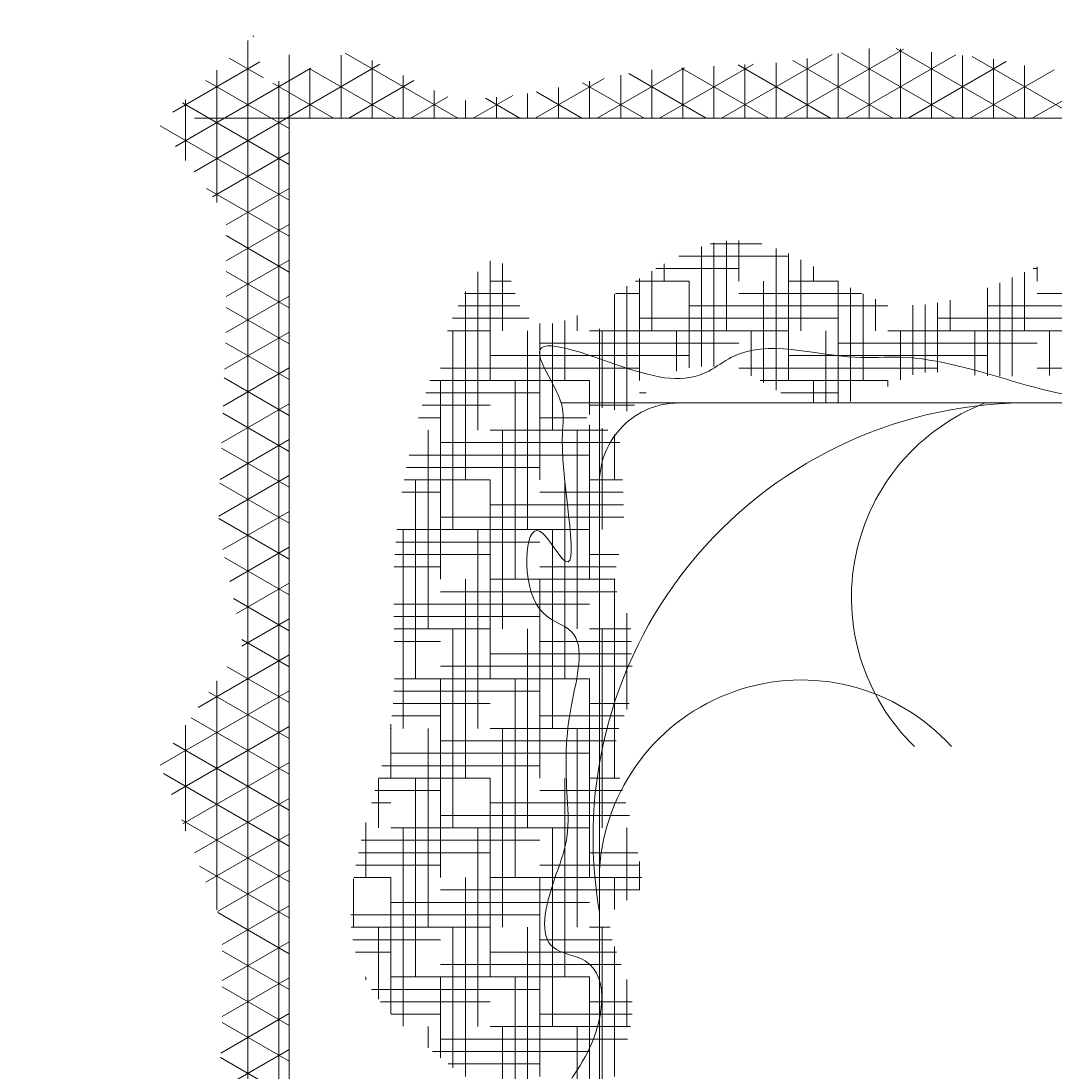
# Model space of a CAD drawing. Units: inches. Extents: x 3731 to 4318, y 1310 to 2388.
# Tile 44 of 57: x 4124 to 4167, y 1999 to 2043. Entities that reach past the tile are written whole.
import ezdxf

# ---------------------------------------------------------------- set-up
doc = ezdxf.new("R2010")
doc.units = ezdxf.units.IN
doc.layers.add('A-ANNO-DIMS', color=2, linetype='Continuous', lineweight=18)
doc.layers.add('A-FURN', color=8, linetype='Continuous', lineweight=13)
doc.styles.get("Standard").update_dxf_attribs({"font": 'arial.ttf'})
doc.dimstyles.get("Standard").update_dxf_attribs({"dimtxt": 0.18, "dimasz": 0.18, "dimexe": 0.18, "dimexo": 0.0625, "dimgap": 0.09, "dimtad": 0, "dimtih": 1, "dimtoh": 1, "dimdec": 4, "dimzin": 0, "dimdsep": 46, "dimtxsty": 'Standard', "dimcen": 0.09, "dimadec": 0, "dimazin": 0, "dimtfac": 1, "dimtdec": 4, "dimtofl": 0, "dimtmove": 0, "dimatfit": 3, "dimfxl": 1, "dimtolj": 1, "dimtzin": 0, "dimarcsym": 0})

# ---------------------------------------------------------------- blocks, each defined once
blk = doc.blocks.new('A$C200C7901')
for p, q in [((2.3121, 1.6596), (2.3121, 0.0201)), ((2, 0.2957), (2, 1.2957)), ((2.0224, 0.9977), (2.0224, 1.1977)), ((2.0224, 0.9977), (2.0224, 1.1977)), ((1.9974, 0.5977), (1.9974, 0.7977)), ((1.9974, 0.5977), (1.9974, 0.7977)), ((2.0724, 0.5977), (2.0724, 0.7977)), ((2.0724, 0.5977), (2.0724, 0.7977)), ((2.1474, 0.5977), (2.1474, 0.7977)), ((2.1474, 0.5977), (2.1474, 0.7977)), ((1.9849, 0.5477), (1.9849, 0.7477)), ((1.9849, 0.5477), (1.9849, 0.7477)), ((2.0599, 0.5477), (2.0599, 0.7477)), ((2.0599, 0.5477), (2.0599, 0.7477)), ((2.1349, 0.5477), (2.1349, 0.7477)), ((2.1349, 0.5477), (2.1349, 0.7477)), ((0.4061, 0.3703), (2.0386, 0.3703)), ((2.4073, 0.0839), (0.9625, 0.0839))]:
    blk.add_line(p, q)
at = {"linetype": 'ByBlock'}
for p, q in [((2.3224, 0.0468), (2.3224, 1.6627)), ((2.3224, 0.0468), (2.3224, 1.6627)), ((2.3537, 0.0056), (2.3537, 1.634)), ((2.3537, 0.0056), (2.3537, 1.634)), ((2.0099, 0.9477), (2.0099, 1.1477)), ((2.0099, 0.9477), (2.0099, 1.1477)), ((2.0849, 0.9477), (2.0849, 1.1477)), ((2.0849, 0.9477), (2.0849, 1.1477)), ((1.9974, 0.8977), (1.9974, 1.0977)), ((1.9974, 0.8977), (1.9974, 1.0977)), ((2.0724, 0.8977), (2.0724, 1.0977)), ((2.0724, 0.8977), (2.0724, 1.0977)), ((2.0974, 0.9977), (2.0974, 1.0909)), ((2.0974, 0.9977), (2.0974, 1.0909)), ((2.3121, 1.0686), (2.3813, 1.0286)), ((2.3121, 1.0686), (2.3813, 1.0286)), ((2.3121, 1.0206), (2.3851, 1.0628)), ((2.3121, 1.0206), (2.3851, 1.0628)), ((1.9849, 0.9171), (1.9849, 1.0477)), ((1.9849, 0.9171), (1.9849, 1.0477)), ((2.0599, 0.8477), (2.0599, 1.0477)), ((2.0599, 0.8477), (2.0599, 1.0477)), ((2.1349, 0.8477), (2.1349, 1.0477)), ((2.1349, 0.8477), (2.1349, 1.0477)), ((2.0599, 1.0352), (2.1523, 1.0352)), ((2.0599, 1.0352), (2.1523, 1.0352)), ((2.1474, 0.8977), (2.1474, 1.0391)), ((2.1474, 0.8977), (2.1474, 1.0391)), ((2.1599, 0.9477), (2.1599, 1.029)), ((2.1599, 0.9477), (2.1599, 1.029)), ((2.3121, 1.0325), (2.3795, 0.9936)), ((2.3121, 1.0325), (2.3795, 0.9936)), ((2.0099, 1.0227), (2.1678, 1.0227)), ((2.0099, 1.0227), (2.1678, 1.0227)), ((2.1724, 0.9977), (2.1724, 1.0189)), ((2.1724, 0.9977), (2.1724, 1.0189)), ((2.3121, 0.9846), (2.3809, 1.0242)), ((2.3121, 0.9846), (2.3809, 1.0242)), ((1.9718, 1.0102), (2.1599, 1.0102)), ((1.9718, 1.0102), (2.1599, 1.0102)), ((1.9688, 0.9977), (2.1099, 0.9977)), ((1.9688, 0.9977), (2.1099, 0.9977)), ((1.9724, 0.9504), (1.9724, 0.9977)), ((1.9724, 0.9504), (1.9724, 0.9977)), ((2.0474, 0.7977), (2.0474, 0.9977)), ((2.0474, 0.7977), (2.0474, 0.9977)), ((2.1224, 0.7977), (2.1224, 0.9977)), ((2.1224, 0.7977), (2.1224, 0.9977)), ((2.1974, 0.7977), (2.1974, 0.9972)), ((2.1974, 0.7977), (2.1974, 0.9972)), ((2.3121, 0.9964), (2.3795, 0.9575)), ((2.3121, 0.9964), (2.3795, 0.9575)), ((1.9671, 0.9852), (2.0599, 0.9852)), ((1.9671, 0.9852), (2.0599, 0.9852)), ((2.1599, 0.9852), (2.2095, 0.9852)), ((2.1599, 0.9852), (2.2095, 0.9852)), ((2.2099, 0.8477), (2.2099, 0.9848)), ((2.2099, 0.8477), (2.2099, 0.9848)), ((2.3121, 0.9485), (2.3795, 0.9874)), ((2.3121, 0.9485), (2.3795, 0.9874)), ((1.9672, 0.9727), (2.0099, 0.9727)), ((1.9672, 0.9727), (2.0099, 0.9727)), ((2.1099, 0.9727), (2.2204, 0.9727)), ((2.1099, 0.9727), (2.2204, 0.9727)), ((2.2224, 0.8977), (2.2224, 0.9702)), ((2.2224, 0.8977), (2.2224, 0.9702)), ((2.0599, 0.9602), (2.2294, 0.9602)), ((2.0599, 0.9602), (2.2294, 0.9602)), ((2.2349, 0.9477), (2.2349, 0.9506)), ((2.2349, 0.9477), (2.2349, 0.9506)), ((2.3121, 0.9603), (2.3795, 0.9215)), ((2.3121, 0.9603), (2.3795, 0.9215)), ((2.3121, 0.9124), (2.3795, 0.9513)), ((2.3121, 0.9124), (2.3795, 0.9513)), ((2.0099, 0.9477), (2.2099, 0.9477)), ((2.0099, 0.9477), (2.2099, 0.9477)), ((2.0349, 0.7477), (2.0349, 0.9477)), ((2.0349, 0.7477), (2.0349, 0.9477)), ((2.1099, 0.7477), (2.1099, 0.9477)), ((2.1099, 0.7477), (2.1099, 0.9477)), ((2.1849, 0.7477), (2.1849, 0.9477)), ((2.1849, 0.7477), (2.1849, 0.9477)), ((1.9781, 0.9352), (2.1599, 0.9352)), ((1.9781, 0.9352), (2.1599, 0.9352)), ((1.9829, 0.9227), (2.1099, 0.9227)), ((1.9829, 0.9227), (2.1099, 0.9227)), ((2.2099, 0.9227), (2.2455, 0.9227)), ((2.2099, 0.9227), (2.2455, 0.9227)), ((2.3121, 0.9243), (2.3838, 0.8829)), ((2.3121, 0.9243), (2.3838, 0.8829)), ((1.9871, 0.9102), (2.0599, 0.9102)), ((1.9871, 0.9102), (2.0599, 0.9102)), ((2.1599, 0.9102), (2.2481, 0.9102)), ((2.1599, 0.9102), (2.2481, 0.9102)), ((2.3121, 0.8763), (2.3795, 0.9152)), ((2.3121, 0.8763), (2.3795, 0.9152)), ((1.9894, 0.8977), (2.0099, 0.8977)), ((1.9894, 0.8977), (2.0099, 0.8977)), ((2.0224, 0.6977), (2.0224, 0.8977)), ((2.0224, 0.6977), (2.0224, 0.8977)), ((2.0974, 0.6977), (2.0974, 0.8977)), ((2.0974, 0.6977), (2.0974, 0.8977)), ((2.1099, 0.8977), (2.2496, 0.8977)), ((2.1099, 0.8977), (2.2496, 0.8977)), ((2.1724, 0.6977), (2.1724, 0.8977)), ((2.1724, 0.6977), (2.1724, 0.8977)), ((2.2474, 0.8489), (2.2474, 0.8977)), ((2.2474, 0.8489), (2.2474, 0.8977)), ((2.3121, 0.8882), (2.4022, 0.8362)), ((2.3121, 0.8882), (2.4022, 0.8362)), ((1.9849, 0.8477), (1.9849, 0.88)), ((1.9849, 0.8477), (1.9849, 0.88)), ((2.0599, 0.8852), (2.2501, 0.8852)), ((2.0599, 0.8852), (2.2501, 0.8852)), ((2.3121, 0.8402), (2.3842, 0.8818)), ((2.3121, 0.8402), (2.3842, 0.8818)), ((2.3849, 0.6497), (2.3849, 0.8801)), ((2.3849, 0.6497), (2.3849, 0.8801)), ((1.9724, 0.7977), (1.9724, 0.8703)), ((1.9724, 0.7977), (1.9724, 0.8703)), ((2.0099, 0.8727), (2.2099, 0.8727)), ((2.0099, 0.8727), (2.2099, 0.8727)), ((1.9599, 0.8317), (1.9599, 0.8604)), ((1.9599, 0.8317), (1.9599, 0.8604)), ((1.9599, 0.8602), (2.1599, 0.8602)), ((1.9599, 0.8602), (2.1599, 0.8602)), ((1.9574, 0.8477), (2.1099, 0.8477)), ((1.9574, 0.8477), (2.1099, 0.8477)), ((2.0099, 0.6477), (2.0099, 0.8477)), ((2.0099, 0.6477), (2.0099, 0.8477)), ((2.0849, 0.6477), (2.0849, 0.8477)), ((2.0849, 0.6477), (2.0849, 0.8477)), ((2.1599, 0.6477), (2.1599, 0.8477)), ((2.1599, 0.6477), (2.1599, 0.8477)), ((2.2099, 0.8477), (2.2472, 0.8477)), ((2.2099, 0.8477), (2.2472, 0.8477)), ((2.2349, 0.7923), (2.2349, 0.8477)), ((2.2349, 0.7923), (2.2349, 0.8477)), ((2.3121, 0.8041), (2.3958, 0.8524)), ((2.3121, 0.8041), (2.3958, 0.8524)), ((2.3121, 0.8521), (2.4205, 0.7895)), ((2.3121, 0.8521), (2.4205, 0.7895)), ((1.9593, 0.8352), (2.0599, 0.8352)), ((1.9593, 0.8352), (2.0599, 0.8352)), ((2.1599, 0.8352), (2.2451, 0.8352)), ((2.1599, 0.8352), (2.2451, 0.8352)), ((1.9615, 0.8227), (2.0099, 0.8227)), ((1.9615, 0.8227), (2.0099, 0.8227)), ((2.1099, 0.8227), (2.2425, 0.8227)), ((2.1099, 0.8227), (2.2425, 0.8227)), ((2.3121, 0.7681), (2.4073, 0.823)), ((2.3121, 0.7681), (2.4073, 0.823)), ((2.3121, 0.816), (2.4384, 0.7431)), ((2.3121, 0.816), (2.4384, 0.7431)), ((2.0599, 0.8102), (2.2396, 0.8102)), ((2.0599, 0.8102), (2.2396, 0.8102)), ((2.0099, 0.7977), (2.2099, 0.7977)), ((2.0099, 0.7977), (2.2099, 0.7977)), ((2.2224, 0.7483), (2.2224, 0.7977)), ((2.2224, 0.7483), (2.2224, 0.7977)), ((2.3121, 0.732), (2.4189, 0.7936)), ((2.3121, 0.732), (2.4189, 0.7936)), ((2.4162, 0.6946), (2.4162, 0.8006)), ((2.4162, 0.6946), (2.4162, 0.8006)), ((1.9699, 0.7852), (2.1599, 0.7852)), ((1.9699, 0.7852), (2.1599, 0.7852)), ((1.9734, 0.7727), (2.1099, 0.7727)), ((1.9734, 0.7727), (2.1099, 0.7727)), ((2.2099, 0.7727), (2.2294, 0.7727)), ((2.2099, 0.7727), (2.2294, 0.7727)), ((2.3121, 0.7799), (2.4287, 0.7126)), ((2.3121, 0.7799), (2.4287, 0.7126)), ((2.3121, 0.6959), (2.4303, 0.7641)), ((2.3121, 0.6959), (2.4303, 0.7641)), ((1.9767, 0.7602), (2.0599, 0.7602)), ((1.9767, 0.7602), (2.0599, 0.7602)), ((2.1599, 0.7602), (2.2258, 0.7602)), ((2.1599, 0.7602), (2.2258, 0.7602)), ((1.9797, 0.7477), (2.0099, 0.7477)), ((1.9797, 0.7477), (2.0099, 0.7477)), ((2.1099, 0.7477), (2.2222, 0.7477)), ((2.1099, 0.7477), (2.2222, 0.7477)), ((2.2099, 0.6933), (2.2099, 0.7477)), ((2.2099, 0.6933), (2.2099, 0.7477)), ((2.3121, 0.7438), (2.4108, 0.6869)), ((2.3121, 0.7438), (2.4108, 0.6869)), ((2.0599, 0.7352), (2.2188, 0.7352)), ((2.0599, 0.7352), (2.2188, 0.7352)), ((2.3121, 0.6598), (2.4417, 0.7346)), ((2.3121, 0.6598), (2.4417, 0.7346)), ((2.0099, 0.7227), (2.2099, 0.7227)), ((2.0099, 0.7227), (2.2099, 0.7227)), ((1.9831, 0.7102), (2.1599, 0.7102)), ((1.9831, 0.7102), (2.1599, 0.7102)), ((2.3121, 0.7078), (2.3929, 0.6611)), ((2.3121, 0.7078), (2.3929, 0.6611)), ((1.9804, 0.6977), (2.1099, 0.6977)), ((1.9804, 0.6977), (2.1099, 0.6977)), ((2.0474, 0.4977), (2.0474, 0.6977)), ((2.0474, 0.4977), (2.0474, 0.6977)), ((2.1224, 0.4977), (2.1224, 0.6977)), ((2.1224, 0.4977), (2.1224, 0.6977)), ((2.1974, 0.4977), (2.1974, 0.6977)), ((2.1974, 0.4977), (2.1974, 0.6977)), ((2.2099, 0.6977), (2.2106, 0.6977)), ((2.2099, 0.6977), (2.2106, 0.6977)), ((1.9724, 0.5818), (1.9724, 0.6786)), ((1.9724, 0.5818), (1.9724, 0.6786)), ((1.9753, 0.6852), (2.0599, 0.6852)), ((1.9753, 0.6852), (2.0599, 0.6852)), ((2.1599, 0.6852), (2.2088, 0.6852)), ((2.1599, 0.6852), (2.2088, 0.6852)), ((2.3121, 0.6237), (2.4036, 0.6765)), ((2.3121, 0.6237), (2.4036, 0.6765)), ((1.97, 0.6727), (2.0099, 0.6727)), ((1.97, 0.6727), (2.0099, 0.6727)), ((2.1099, 0.6727), (2.2075, 0.6727)), ((2.1099, 0.6727), (2.2075, 0.6727)), ((2.3121, 0.6717), (2.3744, 0.6357)), ((2.3121, 0.6717), (2.3744, 0.6357)), ((2.0599, 0.6602), (2.2067, 0.6602)), ((2.0599, 0.6602), (2.2067, 0.6602)), ((2.0099, 0.6477), (2.2062, 0.6477)), ((2.0099, 0.6477), (2.2062, 0.6477)), ((2.0349, 0.4477), (2.0349, 0.6477)), ((2.0349, 0.4477), (2.0349, 0.6477)), ((2.1099, 0.4477), (2.1099, 0.6477)), ((2.1099, 0.4477), (2.1099, 0.6477)), ((2.1849, 0.4477), (2.1849, 0.6477)), ((2.1849, 0.4477), (2.1849, 0.6477)), ((1.9673, 0.6352), (2.1599, 0.6352)), ((1.9673, 0.6352), (2.1599, 0.6352)), ((2.3121, 0.6356), (2.3598, 0.6081)), ((2.3121, 0.6356), (2.3598, 0.6081)), ((1.9678, 0.6227), (2.1099, 0.6227)), ((1.9678, 0.6227), (2.1099, 0.6227)), ((2.3121, 0.5876), (2.3598, 0.6151)), ((2.3121, 0.5876), (2.3598, 0.6151)), ((1.9679, 0.6102), (2.0599, 0.6102)), ((1.9679, 0.6102), (2.0599, 0.6102)), ((2.1599, 0.6102), (2.2064, 0.6102)), ((2.1599, 0.6102), (2.2064, 0.6102)), ((1.9685, 0.5977), (2.0099, 0.5977)), ((1.9685, 0.5977), (2.0099, 0.5977)), ((2.0224, 0.3977), (2.0224, 0.5977)), ((2.0224, 0.3977), (2.0224, 0.5977)), ((2.0974, 0.3977), (2.0974, 0.5977)), ((2.0974, 0.3977), (2.0974, 0.5977)), ((2.1099, 0.5977), (2.2066, 0.5977)), ((2.1099, 0.5977), (2.2066, 0.5977)), ((2.1724, 0.3977), (2.1724, 0.5977)), ((2.1724, 0.3977), (2.1724, 0.5977)), ((2.3121, 0.5995), (2.3682, 0.5671)), ((2.3121, 0.5995), (2.3682, 0.5671)), ((2.0599, 0.5852), (2.2069, 0.5852)), ((2.0599, 0.5852), (2.2069, 0.5852)), ((2.3121, 0.5515), (2.365, 0.5821)), ((2.3121, 0.5515), (2.365, 0.5821)), ((2.0099, 0.5727), (2.207, 0.5727)), ((2.0099, 0.5727), (2.207, 0.5727)), ((1.9827, 0.5602), (2.1599, 0.5602)), ((1.9827, 0.5602), (2.1599, 0.5602)), ((2.3121, 0.5634), (2.3771, 0.5259)), ((2.3121, 0.5634), (2.3771, 0.5259)), ((2.3121, 0.5155), (2.3719, 0.55)), ((2.3121, 0.5155), (2.3719, 0.55)), ((1.9842, 0.5477), (2.1099, 0.5477)), ((1.9842, 0.5477), (2.1099, 0.5477)), ((2.0099, 0.3923), (2.0099, 0.5477)), ((2.0099, 0.3923), (2.0099, 0.5477)), ((2.0849, 0.3477), (2.0849, 0.5477)), ((2.0849, 0.3477), (2.0849, 0.5477)), ((2.1599, 0.3477), (2.1599, 0.5477)), ((2.1599, 0.3477), (2.1599, 0.5477)), ((1.9831, 0.5352), (2.0599, 0.5352)), ((1.9831, 0.5352), (2.0599, 0.5352)), ((2.1599, 0.5352), (2.2065, 0.5352)), ((2.1599, 0.5352), (2.2065, 0.5352)), ((1.9807, 0.5227), (2.0099, 0.5227)), ((1.9807, 0.5227), (2.0099, 0.5227)), ((2.1099, 0.5227), (2.2058, 0.5227)), ((2.1099, 0.5227), (2.2058, 0.5227)), ((2.3121, 0.5273), (2.383, 0.4864)), ((2.3121, 0.5273), (2.383, 0.4864)), ((2.3121, 0.4794), (2.3788, 0.5179)), ((2.3121, 0.4794), (2.3788, 0.5179)), ((2.0599, 0.5102), (2.2049, 0.5102)), ((2.0599, 0.5102), (2.2049, 0.5102)), ((1.9974, 0.3957), (1.9974, 0.4977)), ((1.9974, 0.3957), (1.9974, 0.4977)), ((2.0099, 0.4977), (2.2038, 0.4977)), ((2.0099, 0.4977), (2.2038, 0.4977)), ((2.0724, 0.2977), (2.0724, 0.4977)), ((2.0724, 0.2977), (2.0724, 0.4977)), ((2.1474, 0.2977), (2.1474, 0.4977)), ((2.1474, 0.2977), (2.1474, 0.4977)), ((2.3121, 0.4912), (2.3817, 0.4511)), ((2.3121, 0.4912), (2.3817, 0.4511)), ((1.9755, 0.4852), (2.1599, 0.4852)), ((1.9755, 0.4852), (2.1599, 0.4852)), ((2.3121, 0.4433), (2.383, 0.4842)), ((2.3121, 0.4433), (2.383, 0.4842)), ((1.9757, 0.4727), (2.1099, 0.4727)), ((1.9757, 0.4727), (2.1099, 0.4727)), ((1.9762, 0.4602), (2.0599, 0.4602)), ((1.9762, 0.4602), (2.0599, 0.4602)), ((2.1599, 0.4602), (2.1987, 0.4602)), ((2.1599, 0.4602), (2.1987, 0.4602)), ((2.3121, 0.4552), (2.3803, 0.4158)), ((2.3121, 0.4552), (2.3803, 0.4158)), ((1.9768, 0.4477), (2.0099, 0.4477)), ((1.9768, 0.4477), (2.0099, 0.4477)), ((1.9849, 0.402), (1.9849, 0.4477)), ((1.9849, 0.402), (1.9849, 0.4477)), ((2.0599, 0.2903), (2.0599, 0.4477)), ((2.0599, 0.2903), (2.0599, 0.4477)), ((2.1099, 0.4477), (2.1965, 0.4477)), ((2.1099, 0.4477), (2.1965, 0.4477)), ((2.1349, 0.2582), (2.1349, 0.4477)), ((2.1349, 0.2582), (2.1349, 0.4477)), ((2.3121, 0.4072), (2.3815, 0.4473)), ((2.3121, 0.4072), (2.3815, 0.4473)), ((2.0599, 0.4352), (2.194, 0.4352)), ((2.0599, 0.4352), (2.194, 0.4352)), ((2.0099, 0.4227), (2.1913, 0.4227)), ((2.0099, 0.4227), (2.1913, 0.4227)), ((2.3121, 0.4191), (2.3789, 0.3805)), ((2.3121, 0.4191), (2.3789, 0.3805)), ((1.9797, 0.4102), (2.1599, 0.4102)), ((1.9797, 0.4102), (2.1599, 0.4102)), ((2.3121, 0.3711), (2.3801, 0.4103)), ((2.3121, 0.3711), (2.3801, 0.4103)), ((1.9915, 0.3977), (2.1099, 0.3977)), ((1.9915, 0.3977), (2.1099, 0.3977)), ((2.0474, 0.2905), (2.0474, 0.3977)), ((2.0474, 0.2905), (2.0474, 0.3977)), ((2.1224, 0.2385), (2.1224, 0.3977)), ((2.1224, 0.2385), (2.1224, 0.3977)), ((2.0099, 0.3477), (2.0099, 0.382)), ((2.0099, 0.3477), (2.0099, 0.382)), ((2.0127, 0.3852), (2.0599, 0.3852)), ((2.0127, 0.3852), (2.0599, 0.3852)), ((2.1599, 0.3852), (2.1819, 0.3852)), ((2.1599, 0.3852), (2.1819, 0.3852)), ((2.3121, 0.383), (2.3775, 0.3452)), ((2.3121, 0.383), (2.3775, 0.3452)), ((1.7599, 0.2477), (1.7599, 0.3703)), ((1.7599, 0.2477), (1.7599, 0.3703)), ((1.7724, 0.2977), (1.7724, 0.3703)), ((1.7724, 0.2977), (1.7724, 0.3703)), ((1.7849, 0.3477), (1.7849, 0.3703)), ((1.7849, 0.3477), (1.7849, 0.3703)), ((1.9648, 0.3727), (2.0099, 0.3727)), ((1.9648, 0.3727), (2.0099, 0.3727)), ((1.9724, 0.253), (1.9724, 0.3785)), ((1.9724, 0.253), (1.9724, 0.3785)), ((1.9849, 0.2609), (1.9849, 0.3774)), ((1.9849, 0.2609), (1.9849, 0.3774)), ((1.9974, 0.2977), (1.9974, 0.3753)), ((1.9974, 0.2977), (1.9974, 0.3753)), ((2.1099, 0.3727), (2.1784, 0.3727)), ((2.1099, 0.3727), (2.1784, 0.3727)), ((2.3121, 0.335), (2.3786, 0.3734)), ((2.3121, 0.335), (2.3786, 0.3734)), ((1.7474, 0.2546), (1.7474, 0.3689)), ((1.7474, 0.2546), (1.7474, 0.3689)), ((1.7599, 0.3602), (1.8177, 0.3602)), ((1.7599, 0.3602), (1.8177, 0.3602)), ((1.9532, 0.3602), (1.9599, 0.3602)), ((1.9532, 0.3602), (1.9599, 0.3602)), ((2.0599, 0.3602), (2.1747, 0.3602)), ((2.0599, 0.3602), (2.1747, 0.3602)), ((1.7099, 0.3477), (1.7099, 0.3539)), ((1.7099, 0.3477), (1.7099, 0.3539)), ((1.8224, 0.2148), (1.8224, 0.3575)), ((1.8224, 0.2148), (1.8224, 0.3575)), ((1.8349, 0.2477), (1.8349, 0.3497)), ((1.8349, 0.2477), (1.8349, 0.3497)), ((1.5474, 0.2977), (1.5474, 0.3428)), ((1.5474, 0.2977), (1.5474, 0.3428)), ((1.5849, 0.2443), (1.5849, 0.3434)), ((1.5849, 0.2443), (1.5849, 0.3434)), ((1.5974, 0.2496), (1.5974, 0.3435)), ((1.5974, 0.2496), (1.5974, 0.3435)), ((1.6099, 0.2546), (1.6099, 0.3432)), ((1.6099, 0.2546), (1.6099, 0.3432)), ((1.6224, 0.2977), (1.6224, 0.3424)), ((1.6224, 0.2977), (1.6224, 0.3424)), ((1.6599, 0.2695), (1.6599, 0.3394)), ((1.6599, 0.2695), (1.6599, 0.3394)), ((1.6724, 0.2713), (1.6724, 0.3398)), ((1.6724, 0.2713), (1.6724, 0.3398)), ((1.6849, 0.272), (1.6849, 0.3422)), ((1.6849, 0.272), (1.6849, 0.3422)), ((1.6974, 0.2977), (1.6974, 0.3472)), ((1.6974, 0.2977), (1.6974, 0.3472)), ((1.7099, 0.3477), (1.8383, 0.3477)), ((1.7099, 0.3477), (1.8383, 0.3477)), ((1.7349, 0.2607), (1.7349, 0.3477)), ((1.7349, 0.2607), (1.7349, 0.3477)), ((1.8099, 0.2201), (1.8099, 0.3477)), ((1.8099, 0.2201), (1.8099, 0.3477)), ((1.8474, 0.2977), (1.8474, 0.3432)), ((1.8474, 0.2977), (1.8474, 0.3432)), ((1.9224, 0.2977), (1.9224, 0.3385)), ((1.9224, 0.2977), (1.9224, 0.3385)), ((1.9599, 0.2452), (1.9599, 0.3477)), ((1.9599, 0.2452), (1.9599, 0.3477)), ((2.0099, 0.3477), (2.1708, 0.3477)), ((2.0099, 0.3477), (2.1708, 0.3477)), ((2.0349, 0.2874), (2.0349, 0.3477)), ((2.0349, 0.2874), (2.0349, 0.3477)), ((2.1099, 0.2274), (2.1099, 0.3477)), ((2.1099, 0.2274), (2.1099, 0.3477)), ((2.3121, 0.3469), (2.3761, 0.31)), ((2.3121, 0.3469), (2.3761, 0.31)), ((1.3599, 0.3352), (1.5599, 0.3352)), ((1.3599, 0.3352), (1.5599, 0.3352)), ((1.6599, 0.3352), (1.8599, 0.3352)), ((1.6599, 0.3352), (1.8599, 0.3352)), ((1.8849, 0.2093), (1.8849, 0.3337)), ((1.8849, 0.2093), (1.8849, 0.3337)), ((1.8974, 0.2129), (1.8974, 0.3335)), ((1.8974, 0.2129), (1.8974, 0.3335)), ((1.9099, 0.2477), (1.9099, 0.3349)), ((1.9099, 0.2477), (1.9099, 0.3349)), ((1.9599, 0.3352), (2.1599, 0.3352)), ((1.9599, 0.3352), (2.1599, 0.3352)), ((2.3121, 0.299), (2.3772, 0.3365)), ((2.3121, 0.299), (2.3772, 0.3365)), ((1.6099, 0.3227), (1.8099, 0.3227)), ((1.6099, 0.3227), (1.8099, 0.3227)), ((1.9099, 0.3227), (2.1099, 0.3227)), ((1.9099, 0.3227), (2.1099, 0.3227)), ((1.5599, 0.3102), (1.7599, 0.3102)), ((1.5599, 0.3102), (1.7599, 0.3102)), ((1.8599, 0.3102), (2.0599, 0.3102)), ((1.8599, 0.3102), (2.0599, 0.3102)), ((2.3121, 0.3108), (2.3755, 0.2742)), ((2.3121, 0.3108), (2.3755, 0.2742)), ((1.5099, 0.2977), (1.7099, 0.2977)), ((1.5099, 0.2977), (1.7099, 0.2977)), ((1.5724, 0.2389), (1.5724, 0.2977)), ((1.5724, 0.2389), (1.5724, 0.2977)), ((1.6474, 0.2668), (1.6474, 0.2977)), ((1.6474, 0.2668), (1.6474, 0.2977)), ((1.7224, 0.2658), (1.7224, 0.2977)), ((1.7224, 0.2658), (1.7224, 0.2977)), ((1.7974, 0.2263), (1.7974, 0.2977)), ((1.7974, 0.2263), (1.7974, 0.2977)), ((1.8099, 0.2977), (2.0099, 0.2977)), ((1.8099, 0.2977), (2.0099, 0.2977)), ((1.8724, 0.2072), (1.8724, 0.2977)), ((1.8724, 0.2072), (1.8724, 0.2977)), ((1.9474, 0.2376), (1.9474, 0.2977)), ((1.9474, 0.2376), (1.9474, 0.2977)), ((2.0224, 0.2822), (2.0224, 0.2977)), ((2.0224, 0.2822), (2.0224, 0.2977)), ((2.0974, 0.2299), (2.0974, 0.2977)), ((2.0974, 0.2299), (2.0974, 0.2977)), ((2.1099, 0.2977), (2.153, 0.2977)), ((2.1099, 0.2977), (2.153, 0.2977)), ((2.3121, 0.2629), (2.3757, 0.2996)), ((2.3121, 0.2629), (2.3757, 0.2996)), ((1.4599, 0.2852), (1.6599, 0.2852)), ((1.4599, 0.2852), (1.6599, 0.2852)), ((1.7599, 0.2852), (1.9599, 0.2852)), ((1.7599, 0.2852), (1.9599, 0.2852)), ((2.0708, 0.2852), (2.1478, 0.2852)), ((2.0708, 0.2852), (2.1478, 0.2852)), ((2.3121, 0.2747), (2.3755, 0.2381)), ((2.3121, 0.2747), (2.3755, 0.2381)), ((1.4099, 0.2727), (1.6099, 0.2727)), ((1.4099, 0.2727), (1.6099, 0.2727)), ((1.7099, 0.2727), (1.9099, 0.2727)), ((1.7099, 0.2727), (1.9099, 0.2727)), ((2.08, 0.2727), (2.1422, 0.2727)), ((2.08, 0.2727), (2.1422, 0.2727)), ((1.3599, 0.2602), (1.5599, 0.2602)), ((1.3599, 0.2602), (1.5599, 0.2602)), ((1.7361, 0.2602), (1.8599, 0.2602)), ((1.7361, 0.2602), (1.8599, 0.2602)), ((1.9599, 0.2602), (1.9838, 0.2602)), ((1.9599, 0.2602), (1.9838, 0.2602)), ((2.0848, 0.2602), (2.1359, 0.2602)), ((2.0848, 0.2602), (2.1359, 0.2602)), ((2.3121, 0.2268), (2.3755, 0.2634)), ((2.3121, 0.2268), (2.3755, 0.2634)), ((1.5599, 0.2335), (1.5599, 0.2477)), ((1.5599, 0.2335), (1.5599, 0.2477)), ((1.7599, 0.2477), (1.8099, 0.2477)), ((1.7599, 0.2477), (1.8099, 0.2477)), ((1.7849, 0.2332), (1.7849, 0.2477)), ((1.7849, 0.2332), (1.7849, 0.2477)), ((1.8599, 0.2068), (1.8599, 0.2477)), ((1.8599, 0.2068), (1.8599, 0.2477)), ((1.9099, 0.2477), (1.9639, 0.2477)), ((1.9099, 0.2477), (1.9639, 0.2477)), ((1.9349, 0.2304), (1.9349, 0.2477)), ((1.9349, 0.2304), (1.9349, 0.2477)), ((2.0888, 0.2477), (2.1099, 0.2477)), ((2.0888, 0.2477), (2.1099, 0.2477)), ((1.5599, 0.2352), (1.5638, 0.2352)), ((1.5599, 0.2352), (1.5638, 0.2352)), ((1.8599, 0.2352), (1.9433, 0.2352)), ((1.8599, 0.2352), (1.9433, 0.2352)), ((2.3121, 0.2387), (2.3755, 0.202)), ((2.3121, 0.2387), (2.3755, 0.202)), ((1.8099, 0.2227), (1.9203, 0.2227)), ((1.8099, 0.2227), (1.9203, 0.2227)), ((2.3121, 0.1907), (2.3755, 0.2273)), ((2.3121, 0.1907), (2.3755, 0.2273)), ((1.8368, 0.2102), (1.8884, 0.2102)), ((1.8368, 0.2102), (1.8884, 0.2102)), ((2.3121, 0.2026), (2.3953, 0.1545)), ((2.3121, 0.2026), (2.3953, 0.1545)), ((2.3121, 0.1546), (2.3755, 0.1912)), ((2.3121, 0.1546), (2.3755, 0.1912)), ((2.3121, 0.1665), (2.4419, 0.0916)), ((2.3121, 0.1665), (2.4419, 0.0916)), ((2.3121, 0.1185), (2.3891, 0.163)), ((2.3121, 0.1185), (2.3891, 0.163)), ((2.3849, 0.0355), (2.3849, 0.1686)), ((2.3849, 0.0355), (2.3849, 0.1686)), ((2.2208, 0.0297), (2.4078, 0.1377)), ((2.2208, 0.0297), (2.4078, 0.1377)), ((2.3121, 0.1304), (2.4193, 0.0685)), ((2.3121, 0.1304), (2.4193, 0.0685)), ((2.4162, 0.0655), (2.4162, 0.1264)), ((2.4162, 0.0655), (2.4162, 0.1264)), ((2.2903, 0.0337), (2.4265, 0.1124)), ((2.2903, 0.0337), (2.4265, 0.1124)), ((2.3121, 0.0943), (2.3958, 0.046)), ((2.3121, 0.0943), (2.3958, 0.046)), ((1.4693, 0.0288), (1.5647, 0.0839)), ((1.4693, 0.0288), (1.5647, 0.0839)), ((1.5176, 0.0839), (1.6251, 0.0219)), ((1.5176, 0.0839), (1.6251, 0.0219)), ((1.5427, 0.0351), (1.6272, 0.0839)), ((1.5427, 0.0351), (1.6272, 0.0839)), ((1.5724, 0.0308), (1.5724, 0.0839)), ((1.5724, 0.0308), (1.5724, 0.0839)), ((1.5801, 0.0839), (1.7018, 0.0137)), ((1.5801, 0.0839), (1.7018, 0.0137)), ((1.5911, 0.027), (1.6897, 0.0839)), ((1.5911, 0.027), (1.6897, 0.0839)), ((1.6037, 0.0245), (1.6037, 0.0839)), ((1.6037, 0.0245), (1.6037, 0.0839)), ((1.6349, 0.0208), (1.6349, 0.0839)), ((1.6349, 0.0208), (1.6349, 0.0839)), ((1.6416, 0.0201), (1.7522, 0.0839)), ((1.6416, 0.0201), (1.7522, 0.0839)), ((1.6426, 0.0839), (1.7565, 0.0182)), ((1.6426, 0.0839), (1.7565, 0.0182)), ((1.6662, 0.0175), (1.6662, 0.0839)), ((1.6662, 0.0175), (1.6662, 0.0839)), ((1.6944, 0.0145), (1.8147, 0.0839)), ((1.6944, 0.0145), (1.8147, 0.0839)), ((1.6974, 0.0141), (1.6974, 0.0839)), ((1.6974, 0.0141), (1.6974, 0.0839)), ((1.7051, 0.0839), (1.8054, 0.026)), ((1.7051, 0.0839), (1.8054, 0.026)), ((1.7287, 0.0137), (1.7287, 0.0839)), ((1.7287, 0.0137), (1.7287, 0.0839)), ((1.7599, 0.0187), (1.7599, 0.0839)), ((1.7599, 0.0187), (1.7599, 0.0839)), ((1.7659, 0.0197), (1.8772, 0.0839)), ((1.7659, 0.0197), (1.8772, 0.0839)), ((1.7676, 0.0839), (1.8606, 0.0303)), ((1.7676, 0.0839), (1.8606, 0.0303)), ((1.7912, 0.0237), (1.7912, 0.0839)), ((1.7912, 0.0237), (1.7912, 0.0839)), ((1.8224, 0.0281), (1.8224, 0.0839)), ((1.8224, 0.0281), (1.8224, 0.0839)), ((1.8301, 0.0839), (1.9175, 0.0335)), ((1.8301, 0.0839), (1.9175, 0.0335)), ((1.8452, 0.0294), (1.9397, 0.0839)), ((1.8452, 0.0294), (1.9397, 0.0839)), ((1.8537, 0.0299), (1.8537, 0.0839)), ((1.8537, 0.0299), (1.8537, 0.0839)), ((1.8849, 0.0316), (1.8849, 0.0839)), ((1.8849, 0.0316), (1.8849, 0.0839)), ((1.8926, 0.0839), (1.9706, 0.0389)), ((1.8926, 0.0839), (1.9706, 0.0389)), ((1.9146, 0.0333), (2.0022, 0.0839)), ((1.9146, 0.0333), (2.0022, 0.0839)), ((1.9162, 0.0334), (1.9162, 0.0839)), ((1.9162, 0.0334), (1.9162, 0.0839)), ((1.9474, 0.0352), (1.9474, 0.0839)), ((1.9474, 0.0352), (1.9474, 0.0839)), ((1.9551, 0.0839), (2.017, 0.0482)), ((1.9551, 0.0839), (2.017, 0.0482)), ((1.9787, 0.0405), (1.9787, 0.0839)), ((1.9787, 0.0405), (1.9787, 0.0839)), ((1.9953, 0.0438), (2.0647, 0.0839)), ((1.9953, 0.0438), (2.0647, 0.0839)), ((2.0099, 0.0468), (2.0099, 0.0839)), ((2.0099, 0.0468), (2.0099, 0.0839)), ((2.0176, 0.0839), (2.0634, 0.0575)), ((2.0176, 0.0839), (2.0634, 0.0575)), ((2.0412, 0.053), (2.0412, 0.0839)), ((2.0412, 0.053), (2.0412, 0.0839)), ((2.0724, 0.0592), (2.0724, 0.0839)), ((2.0724, 0.0592), (2.0724, 0.0839)), ((2.0801, 0.0839), (2.1147, 0.0639)), ((2.0801, 0.0839), (2.1147, 0.0639)), ((2.0873, 0.0609), (2.1272, 0.0839)), ((2.0873, 0.0609), (2.1272, 0.0839)), ((2.1037, 0.0627), (2.1037, 0.0839)), ((2.1037, 0.0627), (2.1037, 0.0839)), ((2.1349, 0.0662), (2.1349, 0.0839)), ((2.1349, 0.0662), (2.1349, 0.0839)), ((2.1426, 0.0839), (2.2557, 0.0186)), ((2.1426, 0.0839), (2.2557, 0.0186)), ((2.1526, 0.0625), (2.1897, 0.0839)), ((2.1526, 0.0625), (2.1897, 0.0839)), ((2.1662, 0.056), (2.1662, 0.0839)), ((2.1662, 0.056), (2.1662, 0.0839)), ((2.1867, 0.0461), (2.2522, 0.0839)), ((2.1867, 0.0461), (2.2522, 0.0839)), ((2.1974, 0.041), (2.1974, 0.0839)), ((2.1974, 0.041), (2.1974, 0.0839)), ((2.2051, 0.0839), (2.2913, 0.0342)), ((2.2051, 0.0839), (2.2913, 0.0342)), ((2.2287, 0.0259), (2.2287, 0.0839)), ((2.2287, 0.0259), (2.2287, 0.0839)), ((2.2599, 0.0205), (2.2599, 0.0839)), ((2.2599, 0.0205), (2.2599, 0.0839)), ((2.2676, 0.0839), (2.3285, 0.0488)), ((2.2676, 0.0839), (2.3285, 0.0488)), ((2.2912, 0.0341), (2.2912, 0.0839)), ((2.2912, 0.0341), (2.2912, 0.0839)), ((2.3417, 0.0273), (2.429, 0.0777)), ((2.3417, 0.0273), (2.429, 0.0777)), ((2.338, 0.0433), (2.3723, 0.0235)), ((2.338, 0.0433), (2.3723, 0.0235)), ((2.3476, 0.0017), (2.3488, 0.001)), ((2.3476, 0.0017), (2.3488, 0.001))]:
    blk.add_line(p, q, dxfattribs=at)
for centre, radius, start, end in [((1.5693, 0.8075), 0.4372, 269.0679, 9.9322), ((1.7969, 0.8525), 0.2035, 222.1514, 356.4639), ((1.5372, 0.5659), 0.2094, 290.9415, 45.7647), ((1.92, 0.4503), 0.08, 270, 0)]:
    blk.add_arc(centre, radius, start, end)
blk.add_open_spline([(0.473, 1.2954), (0.4739, 1.2781), (0.4755, 1.2477), (0.5032, 1.2084), (0.4801, 1.1701), (0.4928, 1.1255), (0.4674, 1.0912), (0.4579, 1.0351), (0.501, 0.9724), (0.4311, 0.8832), (0.4902, 0.8637), (0.4843, 0.8288), (0.4774, 0.7906), (0.4625, 0.7457), (0.459, 0.6999), (0.4816, 0.6664), (0.4748, 0.625), (0.4791, 0.5889), (0.4533, 0.5528), (0.4738, 0.5004), (0.4658, 0.4502), (0.4696, 0.3946), (0.4189, 0.3935), (0.4493, 0.3684), (0.4694, 0.3857), (0.4922, 0.3576), (0.5297, 0.3262), (0.5917, 0.3353), (0.6454, 0.3754), (0.7083, 0.3741), (0.7643, 0.3328), (0.826, 0.346), (0.925, 0.3388), (1.0353, 0.3593), (1.1561, 0.3744), (1.2477, 0.3154), (1.3302, 0.3474), (1.4086, 0.3512), (1.5217, 0.3878), (1.6362, 0.3176), (1.7682, 0.3285), (1.8402, 0.3019), (1.9071, 0.3529), (1.9647, 0.3412), (2.0795, 0.2948), (2.0472, 0.3498), (2.0343, 0.3772), (2.0435, 0.43), (2.0109, 0.5782), (2.0746, 0.4643), (2.0805, 0.584), (2.0084, 0.5979), (2.0343, 0.6846), (2.0344, 0.746), (2.0293, 0.8096), (2.0489, 0.8545), (2.0652, 0.9218), (1.9842, 0.9297), (2.0007, 1.0162), (2.0367, 1.0585), (2.0367, 1.1102), (2.0457, 1.1647), (2.0226, 1.2084), (2.0234, 1.2306), (2.0236, 1.2352)], degree=3, knots=[0, 0, 0, 0, 51.660678, 90.967412, 128.902454, 170.303599, 219.852997, 247.834962, 336.321557, 429.35469, 458.821847, 477.222321, 524.135809, 581.038434, 617.839381, 657.146115, 693.947125, 740.178081, 760.753248, 820.731705, 885.133458, 928.777044, 953.563729, 976.574207, 995.553042, 1018.563482, 1064.584401, 1147.951297, 1174.787598, 1266.851571, 1308.018447, 1377.066427, 1441.511314, 1608.245014, 1714.11869, 1792.771707, 1913.247991, 1954.931389, 2029.864445, 2259.189419, 2305.221512, 2429.507982, 2456.344283, 2543.92595, 2627.925037, 2662.96218, 2687.736879, 2719.937755, 2839.540991, 2875.47895, 2953.681041, 2993.270313, 3066.872333, 3154.395764, 3200.397042, 3248.426375, 3312.828127, 3347.881398, 3444.484026, 3481.577522, 3518.665244, 3592.267265, 3644.719162, 3658.519501, 3658.519501, 3658.519501, 3658.519501], dxfattribs=at)
blk = doc.blocks.new('*D38')
at = {"layer": 'A-ANNO-DIMS', "color": 0, "lineweight": -2, "transparency": 16777216}
for p, q in [((4103.271, 2262.382), (4318.341, 2262.382)), ((4318.161, 2262.202), (4318.161, 2103.064)), ((4318.161, 1943.562), (4318.161, 2102.7)), ((4234.271, 1943.382), (4318.341, 1943.382))]:
    blk.add_line(p, q, dxfattribs=at)
at = {"layer": 'A-ANNO-DIMS', "color": 0, "transparency": 16777216}
for points in [[(4318.131, 2262.202), (4318.191, 2262.202), (4318.161, 2262.382)], [(4318.131, 1943.562), (4318.191, 1943.562), (4318.161, 1943.382)]]:
    blk.add_solid(points, dxfattribs=at)
at = {"layer": 'Defpoints', "color": 0, "transparency": 16777216}
for p in [(4103.209, 2262.382), (4318.161, 2262.382), (4234.209, 1943.382)]:
    blk.add_point(p, dxfattribs=at)
at = {"layer": 'A-ANNO-DIMS', "color": 0, "transparency": 16777216, "insert": (4318.161, 2102.882), "char_height": 0.18, "attachment_point": 5}
blk.add_mtext('\\A1;319', dxfattribs=at)

msp = doc.modelspace()

# ---------------------------------------------------------------- block references
at = {"layer": 'A-FURN', "xscale": 41.1071563136412, "yscale": 41.1071563136412, "zscale": 41.1071563136412, "rotation": 180}
msp.add_blockref('A$C200C7901', (4230.145, 2042.037), dxfattribs=at)

# ---------------------------------------------------------------- dimensions: what is measured, and where the dimension line sits
at = {"layer": 'A-ANNO-DIMS'}
dim = msp.add_linear_dim(base=(4318.161, 2262.382), p1=(4234.209, 1943.382), p2=(4103.209, 2262.382), angle=90, dimstyle='Standard', override={"dimdec": 0, "dimlfac": 1, "dimrnd": 0, "dimzin": 0, "dimdsep": 46, "dimlunit": 2}, dxfattribs=at)
dim.commit()
dim.dimension.update_dxf_attribs({"geometry": '*D38', "text_midpoint": (4318.161, 2102.882)})

doc.saveas('drawing.dxf')
